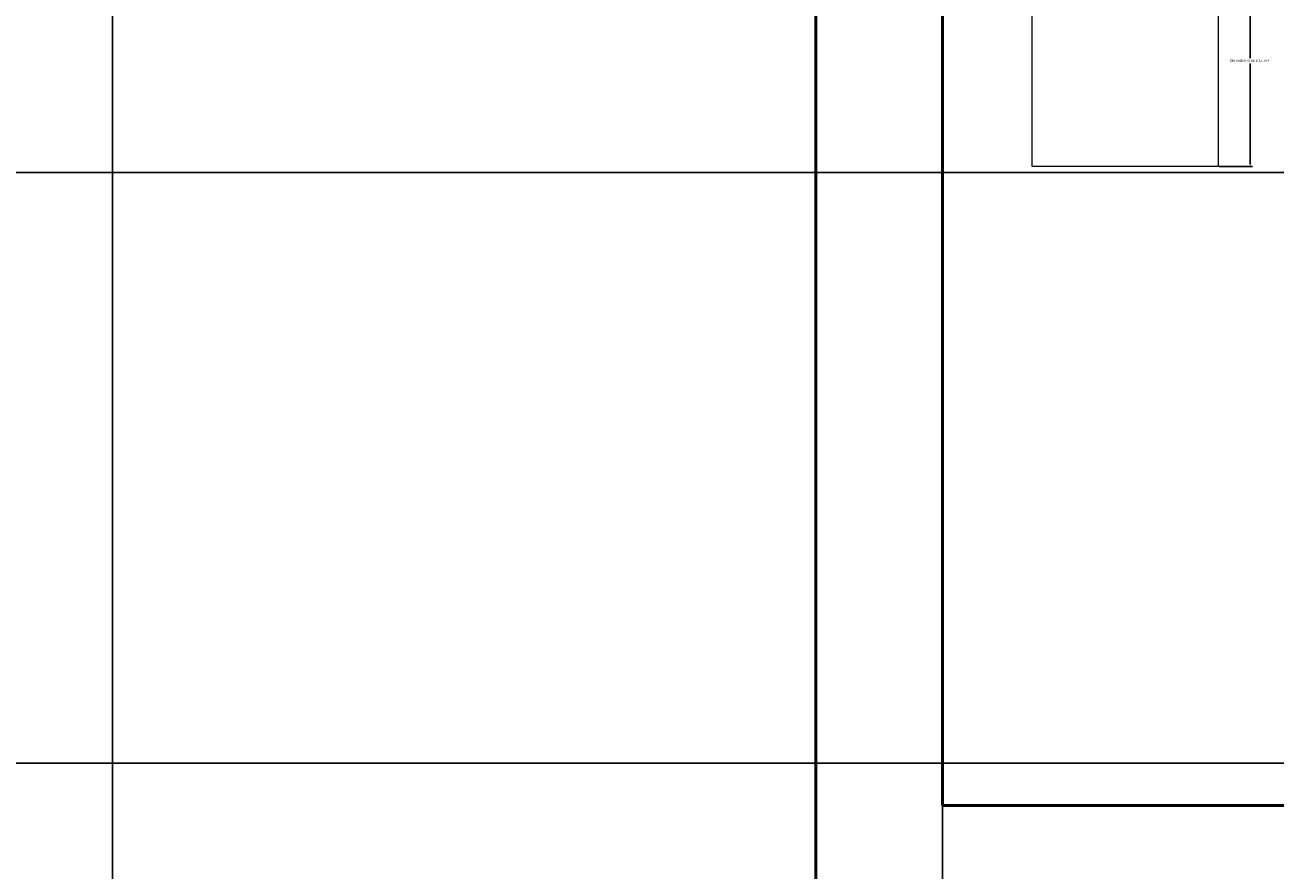
# Model space of a CAD drawing. Units: inches. Extents: x 5375 to 6084, y 16106 to 17259.
# Tile 21 of 32: x 5464 to 5553, y 16872 to 16932. Entities that reach past the tile are written whole.
import ezdxf

# ---------------------------------------------------------------- set-up
doc = ezdxf.new("R2010")
doc.units = ezdxf.units.IN
for name, color, linetype, lineweight in [('A-ANNO-DIMS', 2, 'Continuous', 18), ('FURNITURE', 3, 'Continuous', 18), ('WALL', 6, 'Continuous', 50)]:
    doc.layers.add(name, color=color, linetype=linetype, lineweight=lineweight)
doc.styles.get("Standard").update_dxf_attribs({"font": 'arial.ttf'})
doc.dimstyles.get("Standard").update_dxf_attribs({"dimtxt": 0.18, "dimasz": 0.18, "dimexe": 0.18, "dimexo": 0.0625, "dimgap": 0.09, "dimtad": 0, "dimtih": 1, "dimtoh": 1, "dimdec": 4, "dimzin": 0, "dimdsep": 46, "dimtxsty": 'Standard', "dimcen": 0.09, "dimadec": 0, "dimazin": 0, "dimtfac": 1, "dimtdec": 4, "dimtofl": 0, "dimtmove": 0, "dimatfit": 3, "dimfxl": 1, "dimtolj": 1, "dimtzin": 0, "dimarcsym": 0})

# ---------------------------------------------------------------- blocks, each defined once
blk = doc.blocks.new('NIGHTSTAND-SMALL')
blk.add_lwpolyline([(0, 13.23), (15.042, 13.23), (15.042, 0), (0, 0)], close=True)
blk = doc.blocks.new('*D18')
at = {"layer": 'A-ANNO-DIMS', "color": 0, "lineweight": -2, "transparency": 16777216}
for p, q in [((5549.298, 16937.053), (5551.672, 16937.053)), ((5551.492, 16936.873), (5551.492, 16929.716)), ((5551.492, 16922.192), (5551.492, 16929.349)), ((5549.298, 16922.012), (5551.672, 16922.012))]:
    blk.add_line(p, q, dxfattribs=at)
at = {"layer": 'A-ANNO-DIMS', "color": 0, "transparency": 16777216}
for points in [[(5551.462, 16936.873), (5551.522, 16936.873), (5551.492, 16937.053)], [(5551.462, 16922.192), (5551.522, 16922.192), (5551.492, 16922.012)]]:
    blk.add_solid(points, dxfattribs=at)
at = {"layer": 'Defpoints', "color": 0, "transparency": 16777216}
for p in [(5549.236, 16937.053), (5551.492, 16937.053), (5549.236, 16922.012)]:
    blk.add_point(p, dxfattribs=at)
at = {"layer": 'A-ANNO-DIMS', "color": 0, "transparency": 16777216, "insert": (5551.492, 16929.532), "char_height": 0.18, "attachment_point": 5}
blk.add_mtext('\\A1;SM. NIGHTSTAND 15 TYP.', dxfattribs=at)
blk = doc.blocks.new('*D37')
at = {"layer": 'A-ANNO-DIMS', "color": 0, "lineweight": -2, "transparency": 16777216}
for p, q in [((5520.557, 17206.579), (5375.562, 17206.579)), ((5375.742, 17206.399), (5375.742, 17037.261)), ((5375.742, 16867.759), (5375.742, 17036.897)), ((5520.557, 16867.579), (5375.562, 16867.579))]:
    blk.add_line(p, q, dxfattribs=at)
at = {"layer": 'A-ANNO-DIMS', "color": 0, "transparency": 16777216}
for points in [[(5375.712, 17206.399), (5375.772, 17206.399), (5375.742, 17206.579)], [(5375.712, 16867.759), (5375.772, 16867.759), (5375.742, 16867.579)]]:
    blk.add_solid(points, dxfattribs=at)
at = {"layer": 'Defpoints', "color": 0, "transparency": 16777216}
for p in [(5375.742, 17206.579), (5520.62, 17206.579), (5520.62, 16867.579)]:
    blk.add_point(p, dxfattribs=at)
at = {"layer": 'A-ANNO-DIMS', "color": 0, "transparency": 16777216, "insert": (5375.742, 17037.079), "char_height": 0.18, "attachment_point": 5}
blk.add_mtext('\\A1;339', dxfattribs=at)
blk = doc.blocks.new('*D40')
at = {"layer": 'A-ANNO-DIMS', "color": 0, "lineweight": -2, "transparency": 16777216}
for p, q in [((5529.62, 16876.517), (5529.62, 16106.483)), ((5520.62, 16867.517), (5520.62, 16106.483)), ((5520.8, 16106.663), (5524.971, 16106.663)), ((5529.44, 16106.663), (5525.269, 16106.663))]:
    blk.add_line(p, q, dxfattribs=at)
at = {"layer": 'A-ANNO-DIMS', "color": 0, "transparency": 16777216}
for points in [[(5520.8, 16106.693), (5520.8, 16106.633), (5520.62, 16106.663)], [(5529.44, 16106.693), (5529.44, 16106.633), (5529.62, 16106.663)]]:
    blk.add_solid(points, dxfattribs=at)
at = {"layer": 'Defpoints', "color": 0, "transparency": 16777216}
for p in [(5529.62, 16876.579), (5520.62, 16867.579), (5529.62, 16106.663)]:
    blk.add_point(p, dxfattribs=at)
at = {"layer": 'A-ANNO-DIMS', "color": 0, "transparency": 16777216, "insert": (5525.12, 16106.663), "char_height": 0.18, "attachment_point": 5}
blk.add_mtext('\\A1;9', dxfattribs=at)
blk = doc.blocks.new('*D42')
at = {"layer": 'A-ANNO-DIMS', "color": 0, "lineweight": -2, "transparency": 16777216}
for p, q in [((5826.057, 16921.579), (5375.562, 16921.579)), ((5375.742, 16921.399), (5375.742, 16900.76)), ((5375.742, 16879.759), (5375.742, 16900.399)), ((5826.057, 16879.579), (5375.562, 16879.579))]:
    blk.add_line(p, q, dxfattribs=at)
at = {"layer": 'A-ANNO-DIMS', "color": 0, "transparency": 16777216}
for points in [[(5375.712, 16921.399), (5375.772, 16921.399), (5375.742, 16921.579)], [(5375.712, 16879.759), (5375.772, 16879.759), (5375.742, 16879.579)]]:
    blk.add_solid(points, dxfattribs=at)
at = {"layer": 'Defpoints', "color": 0, "transparency": 16777216}
for p in [(5826.12, 16921.579), (5375.742, 16879.579), (5826.12, 16879.579)]:
    blk.add_point(p, dxfattribs=at)
at = {"layer": 'A-ANNO-DIMS', "color": 0, "transparency": 16777216, "insert": (5375.742, 16900.579), "char_height": 0.18, "attachment_point": 5}
blk.add_mtext('\\A1;42', dxfattribs=at)
blk = doc.blocks.new('*D47')
at = {"layer": 'A-ANNO-DIMS', "color": 0, "lineweight": -2, "transparency": 16777216}
for p, q in [((5470.62, 16603.642), (5470.62, 17259.159)), ((5470.8, 17258.979), (5495.401, 17258.979)), ((5520.44, 17258.979), (5495.839, 17258.979)), ((5520.62, 17206.642), (5520.62, 17259.159))]:
    blk.add_line(p, q, dxfattribs=at)
at = {"layer": 'A-ANNO-DIMS', "color": 0, "transparency": 16777216}
for points in [[(5470.8, 17259.009), (5470.8, 17258.949), (5470.62, 17258.979)], [(5520.44, 17259.009), (5520.44, 17258.949), (5520.62, 17258.979)]]:
    blk.add_solid(points, dxfattribs=at)
at = {"layer": 'Defpoints', "color": 0, "transparency": 16777216}
for p in [(5520.62, 17258.979), (5520.62, 17206.579), (5470.62, 16603.579)]:
    blk.add_point(p, dxfattribs=at)
at = {"layer": 'A-ANNO-DIMS', "color": 0, "transparency": 16777216, "insert": (5495.62, 17258.979), "char_height": 0.18, "attachment_point": 5}
blk.add_mtext('\\A1;50', dxfattribs=at)

msp = doc.modelspace()

# ---------------------------------------------------------------- linework, layer by layer
at = {"layer": 'WALL'}
for p, q in [((5520.6199, 17206.5793), (5520.6199, 16867.5793)), ((5529.6199, 17056.5793), (5529.6199, 16876.5793)), ((5529.6199, 16876.5793), (5702.1199, 16876.5793))]:
    msp.add_line(p, q, dxfattribs=at)

# ---------------------------------------------------------------- block references
at = {"layer": 'FURNITURE', "rotation": 89.99999999998697}
msp.add_blockref('NIGHTSTAND-SMALL', (5549.2363, 16922.0116), dxfattribs=at)

# ---------------------------------------------------------------- dimensions: what is measured, and where the dimension line sits
at = {"layer": 'A-ANNO-DIMS'}
for base, p1, p2, picture, middle in [((5520.6199, 17258.9793), (5470.6199, 16603.5793), (5520.6199, 17206.5793), '*D47', (5495.6199, 17258.9793)), ((5529.6199, 16106.6631), (5520.6199, 16867.5793), (5529.6199, 16876.5793), '*D40', (5525.1199, 16106.6631))]:
    dim = msp.add_linear_dim(base=base, p1=p1, p2=p2, dimstyle='Standard', override={"dimdec": 0, "dimlfac": 1, "dimrnd": 0, "dimzin": 0, "dimdsep": 46, "dimlunit": 2}, dxfattribs=at)
    dim.commit()
    dim.dimension.update_dxf_attribs({"geometry": picture, "text_midpoint": middle})
for base, p1, p2, picture, middle in [((5375.7423, 17206.5793), (5520.6199, 16867.5793), (5520.6199, 17206.5793), '*D37', (5375.7423, 17037.0793)), ((5375.7423, 16879.5793), (5826.1199, 16921.5793), (5826.1199, 16879.5793), '*D42', (5375.7423, 16900.5793))]:
    dim = msp.add_linear_dim(base=base, p1=p1, p2=p2, angle=90, dimstyle='Standard', override={"dimdec": 0, "dimlfac": 1, "dimrnd": 0, "dimzin": 0, "dimdsep": 46, "dimlunit": 2}, dxfattribs=at)
    dim.commit()
    dim.dimension.update_dxf_attribs({"geometry": picture, "text_midpoint": middle})
dim = msp.add_linear_dim(base=(5551.4921, 16937.0532), p1=(5549.2359, 16922.0117), p2=(5549.2359, 16937.0532), angle=90, text='SM. NIGHTSTAND <> TYP.', dimstyle='Standard', override={"dimdec": 0, "dimlfac": 1, "dimrnd": 0, "dimzin": 0, "dimdsep": 46, "dimlunit": 2}, dxfattribs=at)
dim.commit()
dim.dimension.update_dxf_attribs({"geometry": '*D18', "text_midpoint": (5551.4921, 16929.5324)})

doc.saveas('drawing.dxf')
